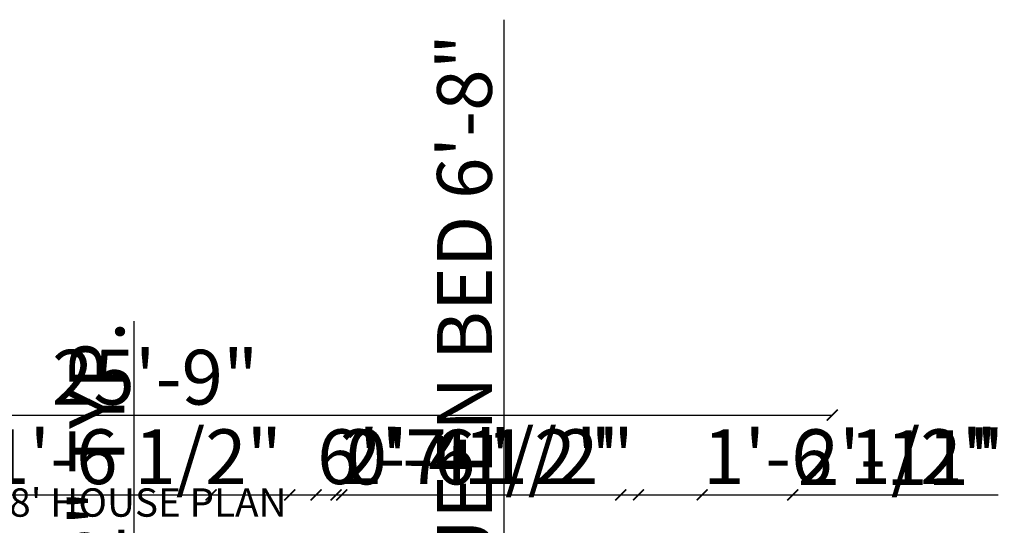
# Model space of a CAD drawing. Units: inches. Extents: x 2419 to 2878, y 1068 to 1713.
# Tile 20 of 20: x 2595 to 2820, y 1598 to 1713. Entities that reach past the tile are written whole.
import ezdxf

# ---------------------------------------------------------------- set-up
doc = ezdxf.new("R2010")
doc.units = ezdxf.units.IN
doc.layers.add('A-ANNO-DIMS', color=2, linetype='Continuous', lineweight=18)
doc.layers.add('A-ANNO-TEXT', color=7, linetype='Continuous', lineweight=25)
doc.styles.get("Standard").update_dxf_attribs({"font": 'arial.ttf'})
doc.dimstyles.new('ISO-25', dxfattribs={"dimtxt": 12.5, "dimasz": 2.5, "dimexe": 1.25, "dimexo": 0.625, "dimtad": 1, "dimdec": 0, "dimlunit": 4, "dimtxsty": 'Standard', "dimblk": 'ARCHTICK', "dimcen": 2.5, "dimse1": 1, "dimse2": 1, "dimclrd": 4, "dimadec": 0, "dimazin": 0, "dimtfac": 1, "dimtdec": 0, "dimtmove": 0, "dimatfit": 3, "dimfxl": 1, "dimarcsym": 0})

# ---------------------------------------------------------------- blocks, each defined once
blk = doc.blocks.new('_ArchTick')
at = {"color": 0, "linetype": 'ByBlock', "const_width": 0.15}
blk.add_lwpolyline([(-0.5, -0.5), (0.5, 0.5)], dxfattribs=at)
blk = doc.blocks.new('*D16')
at = {"layer": 'A-ANNO-DIMS', "color": 0, "lineweight": -2, "transparency": 16777216}
blk.add_line((2471.51, 1623.24), (2780.51, 1623.24), dxfattribs=at)
at = {"layer": 'Defpoints', "color": 0, "transparency": 16777216}
for p in [(2780.51, 1623.24), (2471.51, 1577.81), (2780.51, 1577.81)]:
    blk.add_point(p, dxfattribs=at)
at = {"layer": 'A-ANNO-DIMS', "color": 0, "lineweight": -2, "transparency": 16777216, "xscale": 2.5, "yscale": 2.5, "zscale": 2.5, "rotation": 180}
blk.add_blockref('_ArchTick', (2471.51, 1623.24), dxfattribs=at)
at = {"layer": 'A-ANNO-DIMS', "color": 0, "lineweight": -2, "transparency": 16777216, "xscale": 2.5, "yscale": 2.5, "zscale": 2.5}
blk.add_blockref('_ArchTick', (2780.51, 1623.24), dxfattribs=at)
at = {"layer": 'A-ANNO-DIMS', "color": 0, "transparency": 16777216, "insert": (2626.01, 1630.25), "char_height": 12.5, "attachment_point": 5}
blk.add_mtext('25\'-9"', dxfattribs=at)
blk = doc.blocks.new('*D25')
at = {"layer": 'A-ANNO-DIMS', "color": 4, "lineweight": -2, "transparency": 16777216}
for p, q in [((2621.23, 1565.89), (2621.23, 1644.66)), ((2621.23, 1551.89), (2621.23, 1565.89))]:
    blk.add_line(p, q, dxfattribs=at)
at = {"layer": 'Defpoints', "color": 0, "transparency": 16777216}
for p in [(2619.13, 1565.89), (2621.23, 1565.89), (2619.13, 1551.89)]:
    blk.add_point(p, dxfattribs=at)
at = {"layer": 'A-ANNO-DIMS', "color": 4, "lineweight": -2, "transparency": 16777216, "xscale": 2.5, "yscale": 2.5, "zscale": 2.5}
for p, rotation in [((2621.23, 1565.89), 90), ((2621.23, 1551.89), 270)]:
    blk.add_blockref('_ArchTick', p, dxfattribs=dict(at, rotation=rotation))
at = {"layer": 'A-ANNO-DIMS', "color": 0, "transparency": 16777216, "insert": (2614.32, 1606.52), "char_height": 12.5, "attachment_point": 5, "rotation": 90}
blk.add_mtext('1\'-2" TYP.', dxfattribs=at)
blk = doc.blocks.new('*D30')
at = {"layer": 'A-ANNO-DIMS', "color": 4, "lineweight": -2, "transparency": 16777216}
for p, q in [((2705.68, 1568.81), (2705.68, 1713.47)), ((2705.68, 1488.81), (2705.68, 1568.81))]:
    blk.add_line(p, q, dxfattribs=at)
at = {"layer": 'Defpoints', "color": 0, "transparency": 16777216}
for p in [(2693.68, 1568.81), (2705.68, 1568.81), (2693.68, 1488.81)]:
    blk.add_point(p, dxfattribs=at)
at = {"layer": 'A-ANNO-DIMS', "color": 4, "lineweight": -2, "transparency": 16777216, "xscale": 2.5, "yscale": 2.5, "zscale": 2.5}
for p, rotation in [((2705.68, 1568.81), 90), ((2705.68, 1488.81), 270)]:
    blk.add_blockref('_ArchTick', p, dxfattribs=dict(at, rotation=rotation))
at = {"layer": 'A-ANNO-DIMS', "color": 0, "transparency": 16777216, "insert": (2698.21, 1642.39), "char_height": 12.5, "attachment_point": 5, "rotation": 90}
blk.add_mtext('QUEEN BED 6\'-8"', dxfattribs=at)
blk = doc.blocks.new('*D36')
at = {"layer": 'A-ANNO-DIMS', "color": 4, "lineweight": -2, "transparency": 16777216}
blk.add_line((2656.74, 1605.01), (2736.32, 1605.01), dxfattribs=at)
at = {"layer": 'Defpoints', "color": 0, "transparency": 16777216}
for p in [(2736.32, 1605.01), (2656.74, 1205.81), (2736.32, 1205.81)]:
    blk.add_point(p, dxfattribs=at)
at = {"layer": 'A-ANNO-DIMS', "color": 4, "lineweight": -2, "transparency": 16777216, "xscale": 2.5, "yscale": 2.5, "zscale": 2.5, "rotation": 180}
blk.add_blockref('_ArchTick', (2656.74, 1605.01), dxfattribs=at)
at = {"layer": 'A-ANNO-DIMS', "color": 4, "lineweight": -2, "transparency": 16777216, "xscale": 2.5, "yscale": 2.5, "zscale": 2.5}
blk.add_blockref('_ArchTick', (2736.32, 1605.01), dxfattribs=at)
at = {"layer": 'A-ANNO-DIMS', "color": 0, "transparency": 16777216, "insert": (2696.53, 1612.1), "char_height": 12.5, "attachment_point": 5}
blk.add_mtext('6\'-7 1/2"', dxfattribs=at)
blk = doc.blocks.new('*D37')
at = {"layer": 'A-ANNO-DIMS', "color": 4, "lineweight": -2, "transparency": 16777216}
for p, q in [((2736.32, 1605.01), (2771.51, 1605.01)), ((2771.51, 1605.01), (2818.42, 1605.01))]:
    blk.add_line(p, q, dxfattribs=at)
at = {"layer": 'Defpoints', "color": 0, "transparency": 16777216}
for p in [(2771.51, 1605.01), (2736.32, 1205.81), (2771.51, 1205.81)]:
    blk.add_point(p, dxfattribs=at)
at = {"layer": 'A-ANNO-DIMS', "color": 4, "lineweight": -2, "transparency": 16777216, "xscale": 2.5, "yscale": 2.5, "zscale": 2.5, "rotation": 180}
blk.add_blockref('_ArchTick', (2736.32, 1605.01), dxfattribs=at)
at = {"layer": 'A-ANNO-DIMS', "color": 4, "lineweight": -2, "transparency": 16777216, "xscale": 2.5, "yscale": 2.5, "zscale": 2.5}
blk.add_blockref('_ArchTick', (2771.51, 1605.01), dxfattribs=at)
at = {"layer": 'A-ANNO-DIMS', "color": 0, "transparency": 16777216, "insert": (2796.22, 1611.91), "char_height": 12.5, "attachment_point": 5}
blk.add_mtext('2\'-11"', dxfattribs=at)
blk = doc.blocks.new('*D39')
at = {"layer": 'A-ANNO-DIMS', "color": 4, "lineweight": -2, "transparency": 16777216}
for p, q in [((2662.74, 1605.01), (2668.59, 1605.01)), ((2668.59, 1605.01), (2705.56, 1605.01))]:
    blk.add_line(p, q, dxfattribs=at)
at = {"layer": 'Defpoints', "color": 0, "transparency": 16777216}
for p in [(2668.59, 1605.01), (2662.74, 1165.6), (2668.59, 1165.6)]:
    blk.add_point(p, dxfattribs=at)
at = {"layer": 'A-ANNO-DIMS', "color": 4, "lineweight": -2, "transparency": 16777216, "xscale": 2.5, "yscale": 2.5, "zscale": 2.5, "rotation": 180}
blk.add_blockref('_ArchTick', (2662.74, 1605.01), dxfattribs=at)
at = {"layer": 'A-ANNO-DIMS', "color": 4, "lineweight": -2, "transparency": 16777216, "xscale": 2.5, "yscale": 2.5, "zscale": 2.5}
blk.add_blockref('_ArchTick', (2668.59, 1605.01), dxfattribs=at)
at = {"layer": 'A-ANNO-DIMS', "color": 0, "transparency": 16777216, "insert": (2688.32, 1612.02), "char_height": 12.5, "attachment_point": 5}
blk.add_mtext('0\'-6"', dxfattribs=at)
blk = doc.blocks.new('*D46')
at = {"layer": 'A-ANNO-DIMS', "color": 4, "lineweight": -2, "transparency": 16777216}
for p, q in [((2569.11, 1605.01), (2587.69, 1605.01)), ((2587.69, 1605.01), (2652.62, 1605.01))]:
    blk.add_line(p, q, dxfattribs=at)
at = {"layer": 'Defpoints', "color": 0, "transparency": 16777216}
for p in [(2587.69, 1605.01), (2569.11, 1512.81), (2587.69, 1512.81)]:
    blk.add_point(p, dxfattribs=at)
at = {"layer": 'A-ANNO-DIMS', "color": 4, "lineweight": -2, "transparency": 16777216, "xscale": 2.5, "yscale": 2.5, "zscale": 2.5, "rotation": 180}
blk.add_blockref('_ArchTick', (2569.11, 1605.01), dxfattribs=at)
at = {"layer": 'A-ANNO-DIMS', "color": 4, "lineweight": -2, "transparency": 16777216, "xscale": 2.5, "yscale": 2.5, "zscale": 2.5}
blk.add_blockref('_ArchTick', (2587.69, 1605.01), dxfattribs=at)
at = {"layer": 'A-ANNO-DIMS', "color": 0, "transparency": 16777216, "insert": (2621.41, 1612.1), "char_height": 12.5, "attachment_point": 5}
blk.add_mtext('1\'-6 1/2"', dxfattribs=at)
blk = doc.blocks.new('*D49')
at = {"layer": 'A-ANNO-DIMS', "color": 4, "lineweight": -2, "transparency": 16777216}
for p, q in [((2732.27, 1605.01), (2750.85, 1605.01)), ((2750.85, 1605.01), (2815.78, 1605.01))]:
    blk.add_line(p, q, dxfattribs=at)
at = {"layer": 'Defpoints', "color": 0, "transparency": 16777216}
for p in [(2750.85, 1605.01), (2732.27, 1512.81), (2750.85, 1512.81)]:
    blk.add_point(p, dxfattribs=at)
at = {"layer": 'A-ANNO-DIMS', "color": 4, "lineweight": -2, "transparency": 16777216, "xscale": 2.5, "yscale": 2.5, "zscale": 2.5, "rotation": 180}
blk.add_blockref('_ArchTick', (2732.27, 1605.01), dxfattribs=at)
at = {"layer": 'A-ANNO-DIMS', "color": 4, "lineweight": -2, "transparency": 16777216, "xscale": 2.5, "yscale": 2.5, "zscale": 2.5}
blk.add_blockref('_ArchTick', (2750.85, 1605.01), dxfattribs=at)
at = {"layer": 'A-ANNO-DIMS', "color": 0, "transparency": 16777216, "insert": (2784.57, 1612.1), "char_height": 12.5, "attachment_point": 5}
blk.add_mtext('1\'-6 1/2"', dxfattribs=at)
blk = doc.blocks.new('*D53')
at = {"layer": 'A-ANNO-DIMS', "color": 4, "lineweight": -2, "transparency": 16777216}
for p, q in [((2638.79, 1605.01), (2667.31, 1605.01)), ((2667.31, 1605.01), (2733.63, 1605.01))]:
    blk.add_line(p, q, dxfattribs=at)
at = {"layer": 'Defpoints', "color": 0, "transparency": 16777216}
for p in [(2667.31, 1605.01), (2638.79, 1217.38), (2667.31, 1217.38)]:
    blk.add_point(p, dxfattribs=at)
at = {"layer": 'A-ANNO-DIMS', "color": 4, "lineweight": -2, "transparency": 16777216, "xscale": 2.5, "yscale": 2.5, "zscale": 2.5, "rotation": 180}
blk.add_blockref('_ArchTick', (2638.79, 1605.01), dxfattribs=at)
at = {"layer": 'A-ANNO-DIMS', "color": 4, "lineweight": -2, "transparency": 16777216, "xscale": 2.5, "yscale": 2.5, "zscale": 2.5}
blk.add_blockref('_ArchTick', (2667.31, 1605.01), dxfattribs=at)
at = {"layer": 'A-ANNO-DIMS', "color": 0, "transparency": 16777216, "insert": (2701.72, 1612.1), "char_height": 12.5, "attachment_point": 5}
blk.add_mtext('2\'-4 1/2"', dxfattribs=at)

msp = doc.modelspace()

# ---------------------------------------------------------------- texts
at = {"layer": 'A-ANNO-TEXT'}
msp.add_text('25\'9"X38\' HOUSE PLAN', height=6.4753, dxfattribs=at).set_placement((2561.39, 1600.03))

# ---------------------------------------------------------------- dimensions: what is measured, and where the dimension line sits
at = {"layer": 'A-ANNO-DIMS'}
for base, p1, p2, text, picture, middle in [((2705.68, 1568.81), (2693.68, 1488.81), (2693.68, 1568.81), 'QUEEN BED <>', '*D30', (2698.21, 1642.39)), ((2621.23, 1565.89), (2619.13, 1551.89), (2619.13, 1565.89), '<> TYP.', '*D25', (2614.32, 1606.52))]:
    dim = msp.add_linear_dim(base=base, p1=p1, p2=p2, angle=90, text=text, dimstyle='ISO-25', override={"dimdec": 1, "dimlfac": 1, "dimrnd": 0, "dimzin": 1, "dimdsep": 46, "dimlunit": 4, "dimfrac": 2}, dxfattribs=at)
    dim.commit()
    dim.dimension.update_dxf_attribs({"geometry": picture, "text_midpoint": middle})
for base, p1, p2, override, picture, middle in [((2780.51, 1623.24), (2471.51, 1577.81), (2780.51, 1577.81), {"dimclrd": 0, "dimclre": 0, "dimclrt": 0}, '*D16', (2626.01, 1630.25)), ((2587.69, 1605.01), (2569.11, 1512.81), (2587.69, 1512.81), {"dimdec": 1, "dimlfac": 1, "dimrnd": 0, "dimzin": 1, "dimdsep": 46, "dimlunit": 4, "dimfrac": 2}, '*D46', (2621.41, 1612.1)), ((2667.31, 1605.01), (2638.79, 1217.38), (2667.31, 1217.38), {"dimdec": 1, "dimlfac": 1, "dimrnd": 0, "dimzin": 1, "dimdsep": 46, "dimlunit": 4, "dimfrac": 2}, '*D53', (2701.72, 1612.1)), ((2736.32, 1605.01), (2656.74, 1205.81), (2736.32, 1205.81), {"dimdec": 1, "dimlfac": 1, "dimrnd": 0, "dimzin": 1, "dimdsep": 46, "dimlunit": 4, "dimfrac": 2}, '*D36', (2696.53, 1612.1)), ((2750.85, 1605.01), (2732.27, 1512.81), (2750.85, 1512.81), {"dimdec": 1, "dimlfac": 1, "dimrnd": 0, "dimzin": 1, "dimdsep": 46, "dimlunit": 4, "dimfrac": 2}, '*D49', (2784.57, 1612.1)), ((2668.5856, 1605.013), (2662.7408, 1165.6026), (2668.5856, 1165.6026), {"dimdec": 1, "dimlfac": 1, "dimrnd": 0, "dimzin": 1, "dimdsep": 46, "dimlunit": 4, "dimfrac": 2}, '*D39', (2688.3247, 1612.0201)), ((2771.51, 1605.01), (2736.32, 1205.81), (2771.51, 1205.81), {"dimdec": 1, "dimlfac": 1, "dimrnd": 0, "dimzin": 1, "dimdsep": 46, "dimlunit": 4, "dimfrac": 2}, '*D37', (2796.22, 1611.91))]:
    dim = msp.add_linear_dim(base=base, p1=p1, p2=p2, dimstyle='ISO-25', override=override, dxfattribs=at)
    dim.commit()
    dim.dimension.update_dxf_attribs({"geometry": picture, "text_midpoint": middle})

doc.saveas('drawing.dxf')
